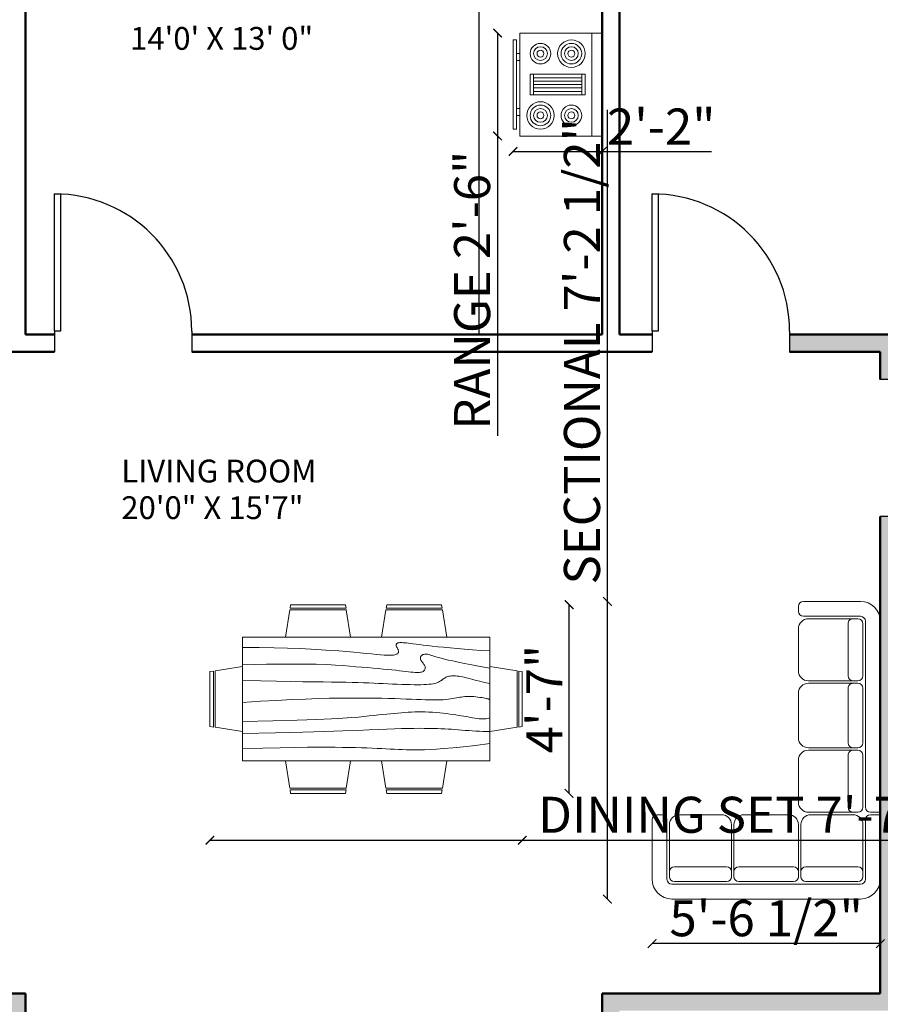
# Model space of a CAD drawing. Units: inches. Extents: x 1549 to 2410, y 1378 to 2139.
# Tile 4 of 6: x 1913 to 2164, y 1654 to 1941. Entities that reach past the tile are written whole.
import ezdxf

# ---------------------------------------------------------------- set-up
doc = ezdxf.new("R2010")
doc.units = ezdxf.units.IN
for name, color, linetype, lineweight in [('A-ANNO-DIMS', 2, 'Continuous', 18), ('A-AREA-IDEN', 7, 'Continuous', 18), ('A-DOOR', 4, 'Continuous', 25), ('A-EQPM', 9, 'Continuous', 18), ('A-FLOR-CASE', 30, 'Continuous', 25), ('A-FURN', 8, 'Continuous', 18), ('A-WALL', 7, 'Continuous', 50)]:
    doc.layers.add(name, color=color, linetype=linetype, lineweight=lineweight)
doc.layers.add('A-WALL-PATT', color=18, linetype='Continuous', lineweight=13, true_color=0x000000)
doc.styles.get("Standard").update_dxf_attribs({"font": 'arial.ttf'})
doc.dimstyles.new('ISO-25', dxfattribs={"dimtxt": 10.5, "dimasz": 2.5, "dimexe": 1.25, "dimexo": 0.625, "dimtad": 1, "dimdec": 0, "dimlunit": 4, "dimtxsty": 'Standard', "dimblk": 'ARCHTICK', "dimcen": 2.5, "dimse1": 1, "dimse2": 1, "dimclrd": 1, "dimclrt": 3, "dimadec": 0, "dimazin": 0, "dimtfac": 1, "dimtdec": 0, "dimtmove": 0, "dimatfit": 3, "dimfxl": 1, "dimarcsym": 0})

# ---------------------------------------------------------------- blocks, each defined once
blk = doc.blocks.new('*U3')
for p, q in [((0, 0), (0, -6)), ((40, 0), (40, -6))]:
    blk.add_line(p, q)
blk.add_lwpolyline([(0, 0), (0, 40), (1.75, 40), (1.75, 0)], close=True)
blk.add_arc((0, 0), 40, 0, 90)
blk = doc.blocks.new('Range-Oven - 30 in top')
for p, q in [((0, -3), (30, -3)), ((12, -6), (18, -6)), ((13, -20), (13, -6)), ((14, -6), (14, -20)), ((15, -20), (15, -6)), ((16, -6), (16, -20)), ((17, -20), (17, -6)), ((18, -20), (12, -20)), ((6, -24), (6, -25)), ((8, -25), (8, -24)), ((22, -25), (22, -24)), ((24, -24), (24, -25))]:
    blk.add_line(p, q)
for points in [[(0, -24), (0, 0), (30, 0), (30, -24)], [(12, -21), (12, -5), (18, -5), (18, -21)], [(2, -26), (2, -25), (28, -25), (28, -26)]]:
    blk.add_lwpolyline(points, close=True)
for centre, radius in [((6, -9), 4), ((6, -9), 3), ((6, -9), 2), ((6, -9), 1), ((24, -9), 3), ((24, -9), 2), ((24, -9), 1), ((24, -18), 4), ((6, -18), 3), ((6, -18), 2), ((6, -18), 1), ((24, -18), 3), ((24, -18), 2), ((24, -18), 1)]:
    blk.add_circle(centre, radius)
blk = doc.blocks.new('Dining Set - 36 x 72 in.')
for p, q in [((-22.2343, 26.00059), (-23.4847, 17.99762)), ((-22.2304, 26), (-5.7608, 26)), ((-22, 27.5), (-22.1562, 26.50042)), ((-5.8416, 26.5), (-22.1534, 26.5)), ((-22, 27.5), (-6, 27.5)), ((-5.8437, 26.49966), (-6, 27.5)), ((-4.5152, 17.99762), (-5.7655, 25.99926)), ((5.7657, 26.00059), (4.5153, 17.99762)), ((5.7696, 26), (22.2392, 26)), ((6, 27.5), (5.8438, 26.50042)), ((22.1584, 26.5), (5.8466, 26.5)), ((6, 27.5), (22, 27.5)), ((22.1563, 26.49966), (22, 27.5)), ((23.4848, 17.99762), (22.2345, 25.99926)), ((36, 18), (-36, 18)), ((-36, 18), (-36, -18)), ((36, -18), (36, 18)), ((-44.0006, 8.23428), (-35.9976, 9.48474)), ((44.0006, 8.23428), (35.9976, 9.48474)), ((-45.5, 8), (-44.5004, 8.15617)), ((-45.5, 8), (-45.5, -8)), ((-44.5, -8.15843), (-44.5, 8.15338)), ((-44, 8.23041), (-44, -8.23915)), ((44, 8.23041), (44, -8.23915)), ((44.5, -8.15843), (44.5, 8.15338)), ((45.5, 8), (44.5005, 8.15617)), ((45.5, 8), (45.5, -8)), ((-44.4997, -8.15631), (-45.5, -8)), ((-35.9976, -9.48476), (-43.9993, -8.2345)), ((35.9976, -9.48476), (43.9993, -8.2345)), ((44.4997, -8.15631), (45.5, -8)), ((-36, -18), (36, -18)), ((-22.2343, -26.0006), (-23.4847, -17.99762)), ((-4.5152, -17.99762), (-5.7655, -25.99928)), ((5.7657, -26.0006), (4.5153, -17.99762)), ((23.4848, -17.99762), (22.2345, -25.99928)), ((-22.2304, -26), (-5.7608, -26)), ((-22, -27.5), (-22.1562, -26.50044)), ((-5.8416, -26.5), (-22.1534, -26.5)), ((-22, -27.5), (-6, -27.5)), ((-5.8437, -26.49967), (-6, -27.5)), ((5.7696, -26), (22.2392, -26)), ((6, -27.5), (5.8438, -26.50044)), ((22.1584, -26.5), (5.8466, -26.5)), ((6, -27.5), (22, -27.5)), ((22.1563, -26.49967), (22, -27.5))]:
    blk.add_line(p, q)
for points in [[(-36, 15), (-31.1772, 14.97754), (-26.8079, 14.91406), (-22.8538, 14.81543), (-19.276, 14.6875), (-16.0362, 14.53613), (-13.0957, 14.36718), (-10.4159, 14.18652), (-7.9583, 14), (-5.6904, 13.81315), (-3.6035, 13.63021), (-1.6954, 13.45508), (0.0365, 13.29166), (1.5945, 13.14388), (2.9811, 13.01562), (4.1988, 12.9108), (5.25, 12.83333), (6.1393, 12.78613), (6.8802, 12.76823), (7.4883, 12.77767), (7.9792, 12.8125), (8.3685, 12.87077), (8.6719, 12.95052), (8.9049, 13.0498), (9.0833, 13.16666), (9.2205, 13.29899), (9.3216, 13.44401), (9.3895, 13.59879), (9.4271, 13.76041), (9.4373, 13.92594), (9.4232, 14.09245), (9.3875, 14.257), (9.3333, 14.41666), (9.2638, 14.56917), (9.1836, 14.71484), (9.0975, 14.85465), (9.0104, 14.98958), (8.9272, 15.1206), (8.8529, 15.2487), (8.7922, 15.37483), (8.75, 15.5), (8.7305, 15.62467), (8.7344, 15.74739), (8.7617, 15.86621), (8.8125, 15.97916), (8.8867, 16.08431), (8.9844, 16.17968), (9.1055, 16.26334), (9.25, 16.33333), (9.4189, 16.38802), (9.6172, 16.42708), (9.8506, 16.45052), (10.125, 16.45833), (10.4463, 16.45052), (10.8203, 16.42708), (11.2529, 16.38802), (11.75, 16.33333), (12.3184, 16.26318), (12.9694, 16.17838), (13.7151, 16.07991), (14.5677, 15.96875), (15.5395, 15.84586), (16.6426, 15.71224), (17.8893, 15.56884), (19.2917, 15.41666), (20.859, 15.25667), (22.5879, 15.08984), (24.4721, 14.91715), (26.5052, 14.73958), (28.6809, 14.5581), (30.9929, 14.3737), (33.4347, 14.18733), (36, 14)], [(-36, 10), (-28.9766, 10.14274), (-23.1725, 10.20442), (-18.4241, 10.19775), (-14.5677, 10.13541), (-11.4399, 10.03011), (-8.877, 9.89453), (-6.7154, 9.74137), (-4.7917, 9.58333), (-2.9698, 9.43082), (-1.2246, 9.28515), (0.4415, 9.14534), (2.026, 9.01041), (3.5266, 8.87939), (4.9408, 8.7513), (6.266, 8.62516), (7.5, 8.5), (8.6411, 8.37549), (9.6914, 8.2539), (10.6538, 8.13818), (11.5312, 8.03125), (12.3267, 7.93603), (13.043, 7.85547), (13.6831, 7.79248), (14.25, 7.75), (14.7471, 7.7303), (15.1797, 7.73307), (15.5537, 7.75732), (15.875, 7.80208), (16.1494, 7.86637), (16.3828, 7.94922), (16.5811, 8.04964), (16.75, 8.16666), (16.8944, 8.29915), (17.0143, 8.44531), (17.1089, 8.60319), (17.1771, 8.77083), (17.218, 8.94629), (17.2305, 9.1276), (17.2137, 9.31282), (17.1667, 9.5), (17.0895, 9.6875), (16.987, 9.875), (16.8649, 10.0625), (16.7292, 10.25), (16.5856, 10.4375), (16.4401, 10.625), (16.2985, 10.8125), (16.1667, 11), (16.05, 11.18733), (15.9518, 11.3737), (15.8752, 11.5581), (15.8229, 11.73958), (15.798, 11.91715), (15.8034, 12.08984), (15.842, 12.25667), (15.9167, 12.41666), (16.0295, 12.56836), (16.1784, 12.70833), (16.3605, 12.83268), (16.5729, 12.9375), (16.8127, 13.01888), (17.0768, 13.07291), (17.3625, 13.0957), (17.6667, 13.08333), (17.9894, 13.03312), (18.3418, 12.94726), (18.7382, 12.82918), (19.1927, 12.68229), (19.7195, 12.51001), (20.3327, 12.31575), (21.0465, 12.10294), (21.875, 11.875), (22.8357, 11.63354), (23.959, 11.37304), (25.2786, 11.08618), (26.8282, 10.76562), (28.6414, 10.40405), (30.752, 9.99414), (33.1936, 9.52856), (36, 9)], [(-36, 5.5), (-30.7157, 5.3348), (-26.069, 5.20963), (-21.9946, 5.11767), (-18.4271, 5.05208), (-15.3009, 5.00602), (-12.5508, 4.97265), (-10.1112, 4.94515), (-7.9167, 4.91666), (-5.909, 4.88167), (-4.0586, 4.83984), (-2.3429, 4.79215), (-0.7396, 4.73958), (0.7739, 4.6831), (2.22, 4.6237), (3.6213, 4.56233), (5, 4.5), (6.373, 4.43782), (7.7344, 4.3776), (9.0723, 4.32129), (10.375, 4.27083), (11.6309, 4.22819), (12.8281, 4.19531), (13.9551, 4.17415), (15, 4.16666), (15.954, 4.17448), (16.819, 4.19791), (17.6001, 4.23698), (18.3021, 4.29166), (18.9299, 4.36198), (19.4883, 4.44791), (19.9823, 4.54948), (20.4167, 4.66666), (20.7969, 4.79899), (21.1302, 4.94401), (21.4245, 5.09879), (21.6875, 5.26041), (21.9271, 5.42594), (22.1511, 5.59245), (22.3672, 5.757), (22.5834, 5.91666), (22.8065, 6.06868), (23.0404, 6.21093), (23.2879, 6.34147), (23.5521, 6.45833), (23.8358, 6.55957), (24.142, 6.64323), (24.4735, 6.70735), (24.8334, 6.75), (25.2235, 6.76969), (25.642, 6.76692), (26.0858, 6.74267), (26.5521, 6.69791), (27.0379, 6.63362), (27.5404, 6.55078), (28.0565, 6.45036), (28.5834, 6.33333), (29.1242, 6.19987), (29.7071, 6.04687), (30.3661, 5.87044), (31.1354, 5.66666), (32.0493, 5.43164), (33.142, 5.16146), (34.4475, 4.85221), (36, 4.5)], [(-36, -1), (-30.7915, -0.6591), (-26.0195, -0.38216), (-21.6519, -0.16284), (-17.6563, 0.00521), (-14.0005, 0.12833), (-10.6523, 0.21289), (-7.5796, 0.26522), (-4.75, 0.29166), (-2.134, 0.29793), (0.2878, 0.28711), (2.5317, 0.26163), (4.6146, 0.22396), (6.5529, 0.17651), (8.3633, 0.12174), (10.0623, 0.06209), (11.6667, 0), (13.1899, -0.06201), (14.6341, -0.1211), (15.9982, -0.17432), (17.2813, -0.21875), (18.4823, -0.25147), (19.6003, -0.26953), (20.6343, -0.27002), (21.5834, -0.25), (22.4481, -0.20768), (23.2357, -0.14584), (23.9549, -0.06836), (24.6146, 0.02083), (25.2235, 0.11784), (25.7904, 0.21875), (26.3241, 0.31966), (26.8334, 0.41666), (27.3265, 0.50618), (27.8099, 0.58593), (28.2894, 0.65397), (28.7709, 0.70833), (29.2601, 0.74707), (29.763, 0.76823), (30.2855, 0.76985), (30.8334, 0.75), (31.4088, 0.70784), (31.9994, 0.64713), (32.589, 0.57275), (33.1615, 0.48958), (33.7008, 0.4025), (34.1908, 0.3164), (34.6153, 0.23616), (34.9584, 0.16666), (35.2099, 0.11165), (35.3848, 0.07031), (35.504, 0.04069), (35.5886, 0.02083), (35.6594, 0.00879), (35.7377, 0.0026), (35.8442, 0.00032), (36, 0)], [(-36, -6.5), (-27.1843, -6.31267), (-20.084, -6.1263), (-14.469, -5.9419), (-10.1094, -5.76042), (-6.7752, -5.58285), (-4.2363, -5.41016), (-2.2629, -5.24333), (-0.625, -5.08334), (0.8708, -4.93099), (2.2715, -4.78646), (3.5872, -4.64974), (4.8281, -4.52084), (6.0046, -4.39974), (7.127, -4.28646), (8.2053, -4.18099), (9.25, -4.08334), (10.2705, -3.99382), (11.2734, -3.91407), (12.2647, -3.84603), (13.25, -3.79167), (14.2354, -3.75293), (15.2266, -3.73177), (16.2295, -3.73015), (17.25, -3.75), (18.2912, -3.79248), (19.3451, -3.85547), (20.4009, -3.93604), (21.4479, -4.03125), (22.4754, -4.13819), (23.4727, -4.25391), (24.4289, -4.37549), (25.3334, -4.5), (26.1785, -4.62492), (26.9694, -4.74935), (27.7145, -4.87281), (28.4219, -4.99479), (29.1, -5.11483), (29.7572, -5.23242), (30.4016, -5.34709), (31.0417, -5.45834), (31.6837, -5.56437), (32.3262, -5.65821), (32.9658, -5.73153), (33.599, -5.77604), (34.2224, -5.78345), (34.8327, -5.74545), (35.4264, -5.65373), (36, -5.5)], [(-36, -10), (-26.4022, -9.81299), (-18.4675, -9.62891), (-11.9839, -9.45069), (-6.7396, -9.28125), (-2.5226, -9.12354), (0.8789, -8.98047), (3.6769, -8.85498), (6.0833, -8.75), (8.2767, -8.66765), (10.3021, -8.60677), (12.1712, -8.56543), (13.8958, -8.54167), (15.4876, -8.53353), (16.9583, -8.53907), (18.3197, -8.55632), (19.5834, -8.58334), (20.7616, -8.61841), (21.8685, -8.66081), (22.9188, -8.71004), (23.9271, -8.76563), (24.9081, -8.82707), (25.8763, -8.89388), (26.8465, -8.96558), (27.8334, -9.04167), (28.8474, -9.12118), (29.8828, -9.20117), (30.93, -9.27824), (31.9792, -9.34896), (33.0205, -9.40991), (34.0443, -9.45768), (35.0407, -9.48885), (36, -9.5)], [(-36, -14.5), (-30.0881, -14.33513), (-25.0332, -14.21224), (-20.7312, -14.12647), (-17.0781, -14.07292), (-13.97, -14.04671), (-11.3027, -14.04297), (-8.9724, -14.05681), (-6.875, -14.08334), (-4.9224, -14.11833), (-3.0905, -14.16016), (-1.3709, -14.20785), (0.2448, -14.26042), (1.7647, -14.3169), (3.1973, -14.3763), (4.5507, -14.43767), (5.8333, -14.5), (7.0554, -14.5621), (8.235, -14.62175), (9.3922, -14.67652), (10.5469, -14.72396), (11.7192, -14.76164), (12.929, -14.78711), (14.1965, -14.79794), (15.5417, -14.79167), (16.9933, -14.76424), (18.6152, -14.70508), (20.4804, -14.60197), (22.6615, -14.44271), (25.2312, -14.21509), (28.2624, -13.9069), (31.8277, -13.50594), (36, -13)]]:
    blk.add_lwpolyline(points)
blk = doc.blocks.new('A$C2AFA021D')
for p, q in [((0.8, 2.3), (0.2, 2.3)), ((0.85, 2.2), (0.85, 2.25)), ((0, 2.1), (0, 0.2)), ((0.15, 0.2), (0.15, 2.1)), ((0.2, 2.15), (0.8, 2.15)), ((0.225, 2.125), (0.275, 2.125)), ((0.75, 2.125), (0.275, 2.125)), ((0.175, 1.55), (0.175, 2.075)), ((0.325, 2.075), (0.325, 1.55)), ((0.85, 1.6), (0.85, 2.025)), ((0.275, 1.5), (0.225, 1.5)), ((0.275, 1.5), (0.75, 1.5)), ((0.175, 0.875), (0.175, 1.425)), ((0.225, 1.475), (0.275, 1.475)), ((0.75, 1.475), (0.275, 1.475)), ((0.325, 1.425), (0.325, 0.875)), ((0.85, 0.925), (0.85, 1.375)), ((0.275, 0.825), (0.225, 0.825)), ((0.225, 0.8), (0.275, 0.8)), ((0.275, 0.825), (0.75, 0.825)), ((0.75, 0.8), (0.275, 0.8)), ((0.975, 0.825), (1.4, 0.825)), ((1.625, 0.825), (2.075, 0.825)), ((2.3, 0.825), (2.725, 0.825)), ((2.9, 0.825), (2.95, 0.825)), ((0.175, 0.225), (0.175, 0.75)), ((0.325, 0.75), (0.325, 0.225)), ((0.85, 0.275), (0.85, 0.7)), ((0.875, 0.275), (0.875, 0.725)), ((1.5, 0.725), (1.5, 0.275)), ((1.525, 0.275), (1.525, 0.725)), ((2.175, 0.725), (2.175, 0.275)), ((2.2, 0.275), (2.2, 0.725)), ((2.825, 0.725), (2.825, 0.275)), ((2.85, 0.2), (2.85, 0.775)), ((3, 0.775), (3, 0.2)), ((1.45, 0.325), (0.925, 0.325)), ((2.125, 0.325), (1.575, 0.325)), ((2.775, 0.325), (2.25, 0.325)), ((0.875, 0.275), (0.875, 0.225)), ((1.5, 0.225), (1.5, 0.275)), ((1.525, 0.275), (1.525, 0.225)), ((2.175, 0.225), (2.175, 0.275)), ((2.2, 0.275), (2.2, 0.225)), ((2.825, 0.225), (2.825, 0.275)), ((0.8, 0.15), (0.2, 0.15)), ((0.275, 0.175), (0.225, 0.175)), ((0.275, 0.175), (0.75, 0.175)), ((0.85, 0), (0.85, 0.1)), ((0.875, 0.1), (0.875, 0)), ((0.925, 0.175), (1.45, 0.175)), ((0.925, 0.15), (2.8, 0.15)), ((1.575, 0.175), (2.125, 0.175)), ((2.25, 0.175), (2.775, 0.175)), ((0.2, 0), (0.85, 0)), ((2.8, 0), (0.875, 0))]:
    blk.add_line(p, q)
for centre, radius, start, end in [((0.2, 2.1), 0.2, 90, 180), ((0.8, 2.25), 0.05, 0, 90), ((0.8, 2.2), 0.05, 270, 0), ((0.2, 2.1), 0.05, 90, 180), ((0.225, 2.075), 0.05, 90, 180), ((0.275, 2.075), 0.05, 0, 90), ((0.75, 2.025), 0.1, 0, 90), ((0.75, 1.6), 0.1, 270, 0), ((0.225, 1.55), 0.05, 180, 270), ((0.275, 1.55), 0.05, 270, 0), ((0.225, 1.425), 0.05, 90, 180), ((0.275, 1.425), 0.05, 0, 90), ((0.75, 1.375), 0.1, 360, 90), ((0.75, 0.925), 0.1, 270, 0), ((0.225, 0.875), 0.05, 180, 270), ((0.225, 0.75), 0.05, 90, 180), ((0.275, 0.875), 0.05, 270, 0), ((0.275, 0.75), 0.05, 0, 90), ((0.75, 0.7), 0.1, 0, 90), ((0.975, 0.725), 0.1, 90, 180), ((1.4, 0.725), 0.1, 0, 90), ((1.625, 0.725), 0.1, 90, 180), ((2.075, 0.725), 0.1, 0, 90), ((2.3, 0.725), 0.1, 90, 180), ((2.725, 0.725), 0.1, 0, 90), ((2.9, 0.775), 0.05, 90, 180), ((2.95, 0.775), 0.05, 0, 90), ((0.925, 0.275), 0.05, 90, 180), ((1.45, 0.275), 0.05, 360, 90), ((1.575, 0.275), 0.05, 90, 180), ((2.125, 0.275), 0.05, 360, 90), ((2.25, 0.275), 0.05, 90, 180), ((2.775, 0.275), 0.05, 360, 90), ((0.2, 0.2), 0.2, 180, 270), ((0.2, 0.2), 0.05, 180, 270), ((0.225, 0.225), 0.05, 180, 270), ((0.275, 0.225), 0.05, 270, 0), ((0.75, 0.275), 0.1, 270, 0), ((0.925, 0.225), 0.05, 180, 270), ((1.45, 0.225), 0.05, 270, 0), ((1.575, 0.225), 0.05, 180, 270), ((2.125, 0.225), 0.05, 270, 0), ((2.25, 0.225), 0.05, 180, 270), ((2.775, 0.225), 0.05, 270, 0), ((2.8, 0.2), 0.2, 270, 0), ((2.8, 0.2), 0.05, 270, 0), ((0.8, 0.1), 0.05, 0, 90), ((0.925, 0.1), 0.05, 90, 180)]:
    blk.add_arc(centre, radius, start, end)
blk = doc.blocks.new('_ArchTick')
at = {"color": 0, "linetype": 'ByBlock', "const_width": 0.15}
blk.add_lwpolyline([(-0.5, -0.5), (0.5, 0.5)], dxfattribs=at)
blk = doc.blocks.new('*D17')
at = {"layer": 'A-ANNO-DIMS', "color": 1, "lineweight": -2, "transparency": 16777216}
for p, q in [((2052.12, 1936.88), (2052.12, 1906.88)), ((2052.12, 1906.88), (2052.12, 1819.52))]:
    blk.add_line(p, q, dxfattribs=at)
at = {"layer": 'Defpoints', "color": 0, "transparency": 16777216}
for p in [(2056.62, 1936.88), (2052.12, 1906.88), (2056.62, 1906.88)]:
    blk.add_point(p, dxfattribs=at)
at = {"layer": 'A-ANNO-DIMS', "color": 1, "lineweight": -2, "transparency": 16777216, "xscale": 2.5, "yscale": 2.5, "zscale": 2.5}
for p, rotation in [((2052.12, 1936.88), 90), ((2052.12, 1906.88), 270)]:
    blk.add_blockref('_ArchTick', p, dxfattribs=dict(at, rotation=rotation))
at = {"layer": 'A-ANNO-DIMS', "color": 3, "transparency": 16777216, "insert": (2046.06, 1861.95), "char_height": 10.5, "attachment_point": 5, "rotation": 90}
blk.add_mtext('RANGE 2\'-6"', dxfattribs=at)
blk = doc.blocks.new('*D18')
at = {"layer": 'A-ANNO-DIMS', "color": 1, "lineweight": -2, "transparency": 16777216}
for p, q in [((2056.62, 1902.38), (2082.62, 1902.38)), ((2082.62, 1902.38), (2114.46, 1902.38))]:
    blk.add_line(p, q, dxfattribs=at)
at = {"layer": 'Defpoints', "color": 0, "transparency": 16777216}
for p in [(2056.62, 1906.88), (2082.62, 1906.88), (2082.62, 1902.38)]:
    blk.add_point(p, dxfattribs=at)
at = {"layer": 'A-ANNO-DIMS', "color": 1, "lineweight": -2, "transparency": 16777216, "xscale": 2.5, "yscale": 2.5, "zscale": 2.5, "rotation": 180}
blk.add_blockref('_ArchTick', (2056.62, 1902.38), dxfattribs=at)
at = {"layer": 'A-ANNO-DIMS', "color": 1, "lineweight": -2, "transparency": 16777216, "xscale": 2.5, "yscale": 2.5, "zscale": 2.5}
blk.add_blockref('_ArchTick', (2082.62, 1902.38), dxfattribs=at)
at = {"layer": 'A-ANNO-DIMS', "color": 3, "transparency": 16777216, "insert": (2099.79, 1908.27), "char_height": 10.5, "attachment_point": 5}
blk.add_mtext('2\'-2"', dxfattribs=at)
blk = doc.blocks.new('*D23')
at = {"layer": 'A-ANNO-DIMS', "color": 1, "lineweight": -2, "transparency": 16777216}
for p, q in [((1968.32, 1701.64), (2059.32, 1701.64)), ((2059.32, 1701.64), (2178.47, 1701.64))]:
    blk.add_line(p, q, dxfattribs=at)
at = {"layer": 'Defpoints', "color": 0, "transparency": 16777216}
for p in [(1968.32, 1715.29), (2059.32, 1715.29), (2059.32, 1701.64)]:
    blk.add_point(p, dxfattribs=at)
at = {"layer": 'A-ANNO-DIMS', "color": 1, "lineweight": -2, "transparency": 16777216, "xscale": 2.5, "yscale": 2.5, "zscale": 2.5, "rotation": 180}
blk.add_blockref('_ArchTick', (1968.32, 1701.64), dxfattribs=at)
at = {"layer": 'A-ANNO-DIMS', "color": 1, "lineweight": -2, "transparency": 16777216, "xscale": 2.5, "yscale": 2.5, "zscale": 2.5}
blk.add_blockref('_ArchTick', (2059.32, 1701.64), dxfattribs=at)
at = {"layer": 'A-ANNO-DIMS', "color": 3, "transparency": 16777216, "insert": (2120.15, 1707.7), "char_height": 10.5, "attachment_point": 5}
blk.add_mtext('DINING SET 7\'-7"', dxfattribs=at)
blk = doc.blocks.new('*D24')
at = {"layer": 'A-ANNO-DIMS', "color": 1, "lineweight": -2, "transparency": 16777216}
blk.add_line((2072.97, 1715.29), (2072.97, 1770.29), dxfattribs=at)
at = {"layer": 'Defpoints', "color": 0, "transparency": 16777216}
for p in [(2059.32, 1770.29), (2072.97, 1770.29), (2059.32, 1715.29)]:
    blk.add_point(p, dxfattribs=at)
at = {"layer": 'A-ANNO-DIMS', "color": 1, "lineweight": -2, "transparency": 16777216, "xscale": 2.5, "yscale": 2.5, "zscale": 2.5}
for p, rotation in [((2072.97, 1770.29), 90), ((2072.97, 1715.29), 270)]:
    blk.add_blockref('_ArchTick', p, dxfattribs=dict(at, rotation=rotation))
at = {"layer": 'A-ANNO-DIMS', "color": 3, "transparency": 16777216, "insert": (2067.09, 1742.79), "char_height": 10.5, "attachment_point": 5, "rotation": 90}
blk.add_mtext('4\'-7"', dxfattribs=at)
blk = doc.blocks.new('*D25')
at = {"layer": 'A-ANNO-DIMS', "color": 1, "lineweight": -2, "transparency": 16777216}
for p, q in [((2084.12, 1771.23), (2084.12, 1914.53)), ((2084.12, 1684.51), (2084.12, 1771.23))]:
    blk.add_line(p, q, dxfattribs=at)
at = {"layer": 'Defpoints', "color": 0, "transparency": 16777216}
for p in [(2084.12, 1771.23), (2097.13, 1771.23), (2097.13, 1684.51)]:
    blk.add_point(p, dxfattribs=at)
at = {"layer": 'A-ANNO-DIMS', "color": 1, "lineweight": -2, "transparency": 16777216, "xscale": 2.5, "yscale": 2.5, "zscale": 2.5}
for p, rotation in [((2084.12, 1771.23), 90), ((2084.12, 1684.51), 270)]:
    blk.add_blockref('_ArchTick', p, dxfattribs=dict(at, rotation=rotation))
at = {"layer": 'A-ANNO-DIMS', "color": 3, "transparency": 16777216, "insert": (2078.06, 1844.13), "char_height": 10.5, "attachment_point": 5, "rotation": 90}
blk.add_mtext('SECTIONAL 7\'-2 1/2"', dxfattribs=at)
blk = doc.blocks.new('*D26')
at = {"layer": 'A-ANNO-DIMS', "color": 1, "lineweight": -2, "transparency": 16777216}
blk.add_line((2163.62, 1671.5), (2097.13, 1671.5), dxfattribs=at)
at = {"layer": 'Defpoints', "color": 0, "transparency": 16777216}
for p in [(2097.13, 1684.51), (2163.62, 1684.51), (2097.13, 1671.5)]:
    blk.add_point(p, dxfattribs=at)
at = {"layer": 'A-ANNO-DIMS', "color": 1, "lineweight": -2, "transparency": 16777216, "xscale": 2.5, "yscale": 2.5, "zscale": 2.5, "rotation": 180}
blk.add_blockref('_ArchTick', (2097.13, 1671.5), dxfattribs=at)
at = {"layer": 'A-ANNO-DIMS', "color": 1, "lineweight": -2, "transparency": 16777216, "xscale": 2.5, "yscale": 2.5, "zscale": 2.5}
blk.add_blockref('_ArchTick', (2163.62, 1671.5), dxfattribs=at)
at = {"layer": 'A-ANNO-DIMS', "color": 3, "transparency": 16777216, "insert": (2130.37, 1677.55), "char_height": 10.5, "attachment_point": 5}
blk.add_mtext('5\'-6 1/2"', dxfattribs=at)
blk = doc.blocks.new('*D50')
at = {"layer": 'A-ANNO-DIMS', "color": 1, "lineweight": -2, "transparency": 16777216}
blk.add_line((1923.02, 1387.76), (1963.02, 1387.76), dxfattribs=at)
at = {"layer": 'Defpoints', "color": 0, "transparency": 16777216}
for p in [(1923.02, 1844.01), (1963.02, 1844.01), (1963.02, 1387.76)]:
    blk.add_point(p, dxfattribs=at)
at = {"layer": 'A-ANNO-DIMS', "color": 1, "lineweight": -2, "transparency": 16777216, "xscale": 2.5, "yscale": 2.5, "zscale": 2.5, "rotation": 180}
blk.add_blockref('_ArchTick', (1923.02, 1387.76), dxfattribs=at)
at = {"layer": 'A-ANNO-DIMS', "color": 1, "lineweight": -2, "transparency": 16777216, "xscale": 2.5, "yscale": 2.5, "zscale": 2.5}
blk.add_blockref('_ArchTick', (1963.02, 1387.76), dxfattribs=at)
at = {"layer": 'A-ANNO-DIMS', "color": 3, "transparency": 16777216, "insert": (1943.02, 1393.75), "char_height": 10.5, "attachment_point": 5}
blk.add_mtext('3\'-4"', dxfattribs=at)
blk = doc.blocks.new('*D52')
at = {"layer": 'A-ANNO-DIMS', "color": 1, "lineweight": -2, "transparency": 16777216}
blk.add_line((2046.65, 1387.76), (2082.62, 1387.76), dxfattribs=at)
at = {"layer": 'Defpoints', "color": 0, "transparency": 16777216}
for p in [(2046.65, 1849.01), (2082.62, 1849.01), (2082.62, 1387.76)]:
    blk.add_point(p, dxfattribs=at)
at = {"layer": 'A-ANNO-DIMS', "color": 1, "lineweight": -2, "transparency": 16777216, "xscale": 2.5, "yscale": 2.5, "zscale": 2.5, "rotation": 180}
blk.add_blockref('_ArchTick', (2046.65, 1387.76), dxfattribs=at)
at = {"layer": 'A-ANNO-DIMS', "color": 1, "lineweight": -2, "transparency": 16777216, "xscale": 2.5, "yscale": 2.5, "zscale": 2.5}
blk.add_blockref('_ArchTick', (2082.62, 1387.76), dxfattribs=at)
at = {"layer": 'A-ANNO-DIMS', "color": 3, "transparency": 16777216, "insert": (2064.64, 1393.75), "char_height": 10.5, "attachment_point": 5}
blk.add_mtext('3\'-0"', dxfattribs=at)
blk = doc.blocks.new('*D54')
at = {"layer": 'A-ANNO-DIMS', "color": 1, "lineweight": -2, "transparency": 16777216}
blk.add_line((2400.7, 1906.88), (2400.7, 1849.01), dxfattribs=at)
at = {"layer": 'Defpoints', "color": 0, "transparency": 16777216}
for p in [(2082.62, 1906.88), (2082.62, 1849.01), (2400.7, 1849.01)]:
    blk.add_point(p, dxfattribs=at)
at = {"layer": 'A-ANNO-DIMS', "color": 1, "lineweight": -2, "transparency": 16777216, "xscale": 2.5, "yscale": 2.5, "zscale": 2.5}
for p, rotation in [((2400.7, 1906.88), 90), ((2400.7, 1849.01), 270)]:
    blk.add_blockref('_ArchTick', p, dxfattribs=dict(at, rotation=rotation))
at = {"layer": 'A-ANNO-DIMS', "color": 3, "transparency": 16777216, "insert": (2394.72, 1877.94), "char_height": 10.5, "attachment_point": 5, "rotation": 90}
blk.add_mtext('4\'-10"', dxfattribs=at)
blk = doc.blocks.new('*D56')
at = {"layer": 'A-ANNO-DIMS', "color": 1, "lineweight": -2, "transparency": 16777216}
for p, q in [((2082.62, 1387.76), (2087.62, 1387.76)), ((2087.62, 1387.76), (2119.28, 1387.76))]:
    blk.add_line(p, q, dxfattribs=at)
at = {"layer": 'Defpoints', "color": 0, "transparency": 16777216}
for p in [(2082.62, 1849.01), (2087.62, 1849.01), (2087.62, 1387.76)]:
    blk.add_point(p, dxfattribs=at)
at = {"layer": 'A-ANNO-DIMS', "color": 1, "lineweight": -2, "transparency": 16777216, "xscale": 2.5, "yscale": 2.5, "zscale": 2.5, "rotation": 180}
blk.add_blockref('_ArchTick', (2082.62, 1387.76), dxfattribs=at)
at = {"layer": 'A-ANNO-DIMS', "color": 1, "lineweight": -2, "transparency": 16777216, "xscale": 2.5, "yscale": 2.5, "zscale": 2.5}
blk.add_blockref('_ArchTick', (2087.62, 1387.76), dxfattribs=at)
at = {"layer": 'A-ANNO-DIMS', "color": 3, "transparency": 16777216, "insert": (2104.7, 1393.75), "char_height": 10.5, "attachment_point": 5}
blk.add_mtext('0\'-5"', dxfattribs=at)
blk = doc.blocks.new('*D59')
at = {"layer": 'A-ANNO-DIMS', "color": 1, "lineweight": -2, "transparency": 16777216}
blk.add_line((2400.7, 1782.99), (2400.7, 1844.01), dxfattribs=at)
at = {"layer": 'Defpoints', "color": 0, "transparency": 16777216}
for p in [(1833.98, 1844.01), (2400.7, 1844.01), (1833.98, 1782.99)]:
    blk.add_point(p, dxfattribs=at)
at = {"layer": 'A-ANNO-DIMS', "color": 1, "lineweight": -2, "transparency": 16777216, "xscale": 2.5, "yscale": 2.5, "zscale": 2.5}
for p, rotation in [((2400.7, 1844.01), 90), ((2400.7, 1782.99), 270)]:
    blk.add_blockref('_ArchTick', p, dxfattribs=dict(at, rotation=rotation))
at = {"layer": 'A-ANNO-DIMS', "color": 3, "transparency": 16777216, "insert": (2394.72, 1813.5), "char_height": 10.5, "attachment_point": 5, "rotation": 90}
blk.add_mtext('5\'-1"', dxfattribs=at)
blk = doc.blocks.new('*D60')
at = {"layer": 'A-ANNO-DIMS', "color": 1, "lineweight": -2, "transparency": 16777216}
blk.add_line((2400.7, 1657.01), (2400.7, 1709.88), dxfattribs=at)
at = {"layer": 'Defpoints', "color": 0, "transparency": 16777216}
for p in [(1870.93, 1709.88), (2400.7, 1709.88), (1870.93, 1657.01)]:
    blk.add_point(p, dxfattribs=at)
at = {"layer": 'A-ANNO-DIMS', "color": 1, "lineweight": -2, "transparency": 16777216, "xscale": 2.5, "yscale": 2.5, "zscale": 2.5}
for p, rotation in [((2400.7, 1709.88), 90), ((2400.7, 1657.01), 270)]:
    blk.add_blockref('_ArchTick', p, dxfattribs=dict(at, rotation=rotation))
at = {"layer": 'A-ANNO-DIMS', "color": 3, "transparency": 16777216, "insert": (2394.74, 1683.45), "char_height": 10.5, "attachment_point": 5, "rotation": 90}
blk.add_mtext('4\'-5"', dxfattribs=at)

msp = doc.modelspace()

# ---------------------------------------------------------------- hatches: boundary and pattern name
at = {"layer": 'A-WALL-PATT'}
h = msp.add_hatch(color=256, dxfattribs=at)
h.dxf.hatch_style = 1
h.paths.add_polyline_path([(1760, 2069.01), (1688.62, 2069.01), (1688.62, 2003.68), (1697.62, 2003.68), (1697.62, 2060.01), (1760, 2060.01)])
h.paths.add_polyline_path([(2309.62, 2069.01), (1807.68, 2069.01), (1807.68, 2060.01), (1909.62, 2060.01), (1909.62, 2040.27), (1914.62, 2040.27), (1914.62, 2060.01), (2082.62, 2060.01), (2082.62, 2043.41), (2087.62, 2043.41), (2087.62, 2060.01), (2300.62, 2060.01), (2300.62, 2006.22), (2309.62, 2006.22)])
h.paths.add_polyline_path([(1914.62, 1607.36), (1909.62, 1607.36), (1909.62, 1437.01), (1914.62, 1437.01)])
h.paths.add_polyline_path([(1697.62, 1536.06), (1688.62, 1536.06), (1688.62, 1428.01), (1745.28, 1428.01), (1745.28, 1437.01), (1697.62, 1437.01)])
h.paths.add_polyline_path([(2130.61, 1437.01), (2082.62, 1437.01), (2082.62, 1428.01), (2130.61, 1428.01)])
h.paths.add_polyline_path([(2309.62, 1544.51), (2302.25, 1544.51), (2302.25, 1524.81), (2300.62, 1524.81), (2300.62, 1523.51), (2302.17, 1523.51), (2302.17, 1503.88), (2300.62, 1503.88), (2300.62, 1437.01), (2193.34, 1437.01), (2193.34, 1428.01), (2309.62, 1428.01)])
h.paths.add_polyline_path([(2309.62, 1708.66), (2300.62, 1708.66), (2300.62, 1657.01), (2293.7, 1657.01), (2293.7, 1652.01), (2300.62, 1652.01), (2300.62, 1611.18), (2302.17, 1611.18), (2302.17, 1597.64), (2309.62, 1597.64)])
h.paths.add_polyline_path([(2309.62, 1777.38), (2300.62, 1777.38), (2300.62, 1737.9), (2309.62, 1737.9)])
h.paths.add_polyline_path([(2300.62, 1757.01), (2168.62, 1757.01), (2168.62, 1795.96), (2163.62, 1795.96), (2163.62, 1657.01), (2082.62, 1657.01), (2082.62, 1641.99), (2087.62, 1641.99), (2087.62, 1652.01), (2253.7, 1652.01), (2253.7, 1657.01), (2168.62, 1657.01), (2168.62, 1752.01), (2300.62, 1752.01)])
h.paths.add_polyline_path([(2309.62, 1957.79), (2300.62, 1957.79), (2300.62, 1935.33), (2300.62, 1824.93), (2309.62, 1824.93)])
h.paths.add_polyline_path([(2300.62, 1849.01), (2137.17, 1849.01), (2137.17, 1844.01), (2163.62, 1844.01), (2163.62, 1835.96), (2168.62, 1835.96), (2168.62, 1844.01), (2300.62, 1844.01)])
h.paths.add_polyline_path([(2211.06, 1800.23), (2261.76, 1800.23), (2261.76, 1810.41), (2211.06, 1810.41)], flags=9)
h.paths.add_polyline_path([(2211.1, 1811.05), (2239.18, 1811.05), (2239.18, 1821.02), (2211.1, 1821.02)], flags=9)
h.paths.add_polyline_path([(2187.84, 1718.73), (2233.38, 1718.73), (2233.38, 1728.91), (2187.84, 1728.91)], flags=25)
h.paths.add_polyline_path([(2187.88, 1729.56), (2215.96, 1729.56), (2215.96, 1739.52), (2187.88, 1739.52)], flags=25)
h.paths.add_polyline_path([(1720.01, 1609.74), (1775.87, 1609.74), (1775.87, 1619.93), (1720.01, 1619.93)], flags=9)
h.paths.add_polyline_path([(1719.99, 1620.4), (1782.23, 1620.4), (1782.23, 1630.72), (1719.99, 1630.72)], flags=9)
h.paths.add_polyline_path([(2092.97, 1541.04), (2148.83, 1541.04), (2148.83, 1551.23), (2092.97, 1551.23)], flags=9)
h.paths.add_polyline_path([(2092.94, 1551.69), (2155.19, 1551.69), (2155.19, 1562.02), (2092.94, 1562.02)], flags=9)
h.paths.add_polyline_path([(1759.73, 1747.67), (1815.59, 1747.67), (1815.59, 1757.85), (1759.73, 1757.85)], flags=9)
h.paths.add_polyline_path([(1759.71, 1758.32), (1790.48, 1758.32), (1790.48, 1768.63), (1759.71, 1768.63)], flags=9)
h.paths.add_polyline_path([(1940.79, 1793.43), (1996.65, 1793.43), (1996.65, 1803.61), (1940.79, 1803.61)], flags=9)
h.paths.add_polyline_path([(1940.77, 1804.08), (2006.11, 1804.08), (2006.11, 1814.4), (1940.77, 1814.4)], flags=9)
h.paths.add_polyline_path([(2094.62, 1963.23), (2150.43, 1963.23), (2150.43, 1973.25), (2094.62, 1973.25)], flags=9)
h.paths.add_polyline_path([(2094.57, 1973.75), (2156.81, 1973.75), (2156.81, 1984.07), (2094.57, 1984.07)], flags=9)
h.paths.add_polyline_path([(1943.36, 1930.19), (2000.28, 1930.19), (2000.28, 1940.37), (1943.36, 1940.37)], flags=9)
h.paths.add_polyline_path([(1943.34, 1940.85), (1987.53, 1940.85), (1987.53, 1951.15), (1943.34, 1951.15)], flags=9)
h.paths.add_polyline_path([(1803.94, 1971.5), (1857.22, 1971.5), (1857.22, 1981.68), (1803.94, 1981.68)], flags=9)
h.paths.add_polyline_path([(1803.92, 1982.16), (1866.16, 1982.16), (1866.16, 1992.47), (1803.92, 1992.47)], flags=9)
h = msp.add_hatch(color=256, dxfattribs=at)
h.dxf.hatch_style = 1
h.paths.add_polyline_path([(1697.62, 1844.01), (1688.62, 1844.01), (1688.62, 1657.01), (1697.62, 1657.01)])
h.paths.add_polyline_path([(1697.62, 1955.9), (1688.62, 1955.9), (1688.62, 1844.01), (1697.62, 1844.01), (1867.86, 1844.01), (1867.86, 1849.01), (1697.62, 1849.01)])
h.paths.add_polyline_path([(1697.62, 1652.01), (1909.62, 1652.01), (1909.62, 1647.36), (1914.62, 1647.36), (1914.62, 1657.01), (1697.62, 1657.01), (1688.62, 1657.01), (1688.62, 1584.55), (1697.62, 1584.55)])
h.paths.add_polyline_path([(2087.62, 1601.99), (2082.62, 1601.99), (2082.62, 1437.01), (2087.62, 1437.01)])
h.paths.add_polyline_path([(1981.52, 1547.01), (1914.62, 1547.01), (1914.62, 1540.24), (1981.52, 1540.24)])
h.paths.add_polyline_path([(2082.62, 1547.01), (2061.69, 1547.01), (2061.69, 1540.24), (2082.62, 1540.24)])

# ---------------------------------------------------------------- linework, layer by layer
at = {"layer": 'A-FLOR-CASE'}
msp.add_line((2046.65, 1973.56), (2046.65, 1849.01), dxfattribs=at)
at = {"layer": 'A-WALL'}
for p, q in [((2087.62, 1849.01), (2087.62, 2060.01)), ((1914.62, 1849.01), (1914.62, 2001.66)), ((2082.62, 1849.01), (2082.62, 2001.66)), ((1914.62, 1849.01), (1923.02, 1849.01)), ((1963.02, 1849.01), (2082.62, 1849.01)), ((2087.62, 1849.01), (2097.17, 1849.01)), ((2137.17, 1849.01), (2300.62, 1849.01)), ((1907.86, 1844.01), (1923.02, 1844.01)), ((1963.02, 1844.01), (2097.17, 1844.01)), ((2137.17, 1844.01), (2163.62, 1844.01)), ((2163.62, 1844.01), (2163.62, 1835.96)), ((2163.62, 1795.96), (2163.62, 1657.01)), ((1697.62, 1657.01), (1914.62, 1657.01)), ((1914.62, 1647.36), (1914.62, 1657.01)), ((2082.62, 1657.01), (2163.62, 1657.01)), ((2082.62, 1641.99), (2082.62, 1657.01))]:
    msp.add_line(p, q, dxfattribs=at)

# ---------------------------------------------------------------- block references
at = {"layer": 'A-DOOR'}
for p in [(1923.02, 1850.01), (2097.17, 1850.01)]:
    msp.add_blockref('*U3', p, dxfattribs=at)
at = {"layer": 'A-DOOR', "rotation": 270}
msp.add_blockref('*U3', (2169.62, 1835.96), dxfattribs=at)
at = {"layer": 'A-EQPM', "rotation": 270}
msp.add_blockref('Range-Oven - 30 in top', (2082.62, 1936.88), dxfattribs=at)
at = {"layer": 'A-FURN', "xscale": 28.90947709907207, "yscale": 28.90947709907207, "zscale": 28.90947709907207, "rotation": 90}
msp.add_blockref('A$C2AFA021D', (2163.62, 1684.51), dxfattribs=at)
at = {"layer": 'A-FURN'}
msp.add_blockref('Dining Set - 36 x 72 in.', (2013.82, 1742.79), dxfattribs=at)

# ---------------------------------------------------------------- texts
at = {"layer": 'A-AREA-IDEN'}
for s, p in [('14\'0\' X 13\' 0"', (1945.06, 1932)), ('LIVING ROOM', (1942.49, 1805.91)), ('20\'0" X 15\'7"', (1942.49, 1795.24))]:
    msp.add_text(s, height=6.6455, dxfattribs=at).set_placement(p)

# ---------------------------------------------------------------- dimensions: what is measured, and where the dimension line sits
at = {"layer": 'A-ANNO-DIMS'}
for base, p1, p2, angle, text, picture, middle in [((2052.12, 1906.88), (2056.62, 1936.88), (2056.62, 1906.88), 270, 'RANGE <>', '*D17', (2046.06, 1861.95)), ((2084.12, 1771.23), (2097.13, 1684.51), (2097.13, 1771.23), 90, 'SECTIONAL <>', '*D25', (2078.06, 1844.13))]:
    dim = msp.add_linear_dim(base=base, p1=p1, p2=p2, angle=angle, text=text, dimstyle='ISO-25', override={"dimdec": 1, "dimlfac": 1, "dimrnd": 0, "dimzin": 1, "dimdsep": 46, "dimlunit": 4, "dimfrac": 2}, dxfattribs=at)
    dim.commit()
    dim.dimension.update_dxf_attribs({"geometry": picture, "text_midpoint": middle})
for base, p1, p2, picture, middle in [((2082.62, 1902.38), (2056.62, 1906.88), (2082.62, 1906.88), '*D18', (2099.79, 1908.27)), ((2082.62, 1387.76), (2046.65, 1849.01), (2082.62, 1849.01), '*D52', (2064.64, 1393.75)), ((2087.62, 1387.76), (2082.62, 1849.01), (2087.62, 1849.01), '*D56', (2104.7, 1393.75)), ((1963.02, 1387.76), (1923.02, 1844.01), (1963.02, 1844.01), '*D50', (1943.02, 1393.75))]:
    dim = msp.add_linear_dim(base=base, p1=p1, p2=p2, dimstyle='ISO-25', override={"dimdec": 1, "dimlfac": 1, "dimrnd": 0, "dimzin": 1, "dimdsep": 46, "dimlunit": 4, "dimfrac": 2}, dxfattribs=at)
    dim.commit()
    dim.dimension.update_dxf_attribs({"geometry": picture, "text_midpoint": middle})
for base, p1, p2, angle, picture, middle in [((2400.7, 1849.01), (2082.62, 1906.88), (2082.62, 1849.01), 90, '*D54', (2394.72, 1877.94)), ((2400.7, 1844.01), (1833.98, 1782.99), (1833.98, 1844.01), 90, '*D59', (2394.72, 1813.5)), ((2072.97, 1770.29), (2059.32, 1715.29), (2059.32, 1770.29), 90, '*D24', (2067.09, 1742.79)), ((2400.7, 1709.88), (1870.93, 1657.01), (1870.93, 1709.88), 90, '*D60', (2394.74, 1683.45)), ((2097.13, 1671.5), (2163.62, 1684.51), (2097.13, 1684.51), 180, '*D26', (2130.37, 1677.55))]:
    dim = msp.add_linear_dim(base=base, p1=p1, p2=p2, angle=angle, dimstyle='ISO-25', override={"dimdec": 1, "dimlfac": 1, "dimrnd": 0, "dimzin": 1, "dimdsep": 46, "dimlunit": 4, "dimfrac": 2}, dxfattribs=at)
    dim.commit()
    dim.dimension.update_dxf_attribs({"geometry": picture, "text_midpoint": middle})
dim = msp.add_linear_dim(base=(2059.32, 1701.64), p1=(1968.32, 1715.29), p2=(2059.32, 1715.29), text='DINING SET <>', dimstyle='ISO-25', override={"dimdec": 1, "dimlfac": 1, "dimrnd": 0, "dimzin": 1, "dimdsep": 46, "dimlunit": 4, "dimfrac": 2}, dxfattribs=at)
dim.commit()
dim.dimension.update_dxf_attribs({"geometry": '*D23', "text_midpoint": (2120.15, 1707.7)})

doc.saveas('drawing.dxf')
